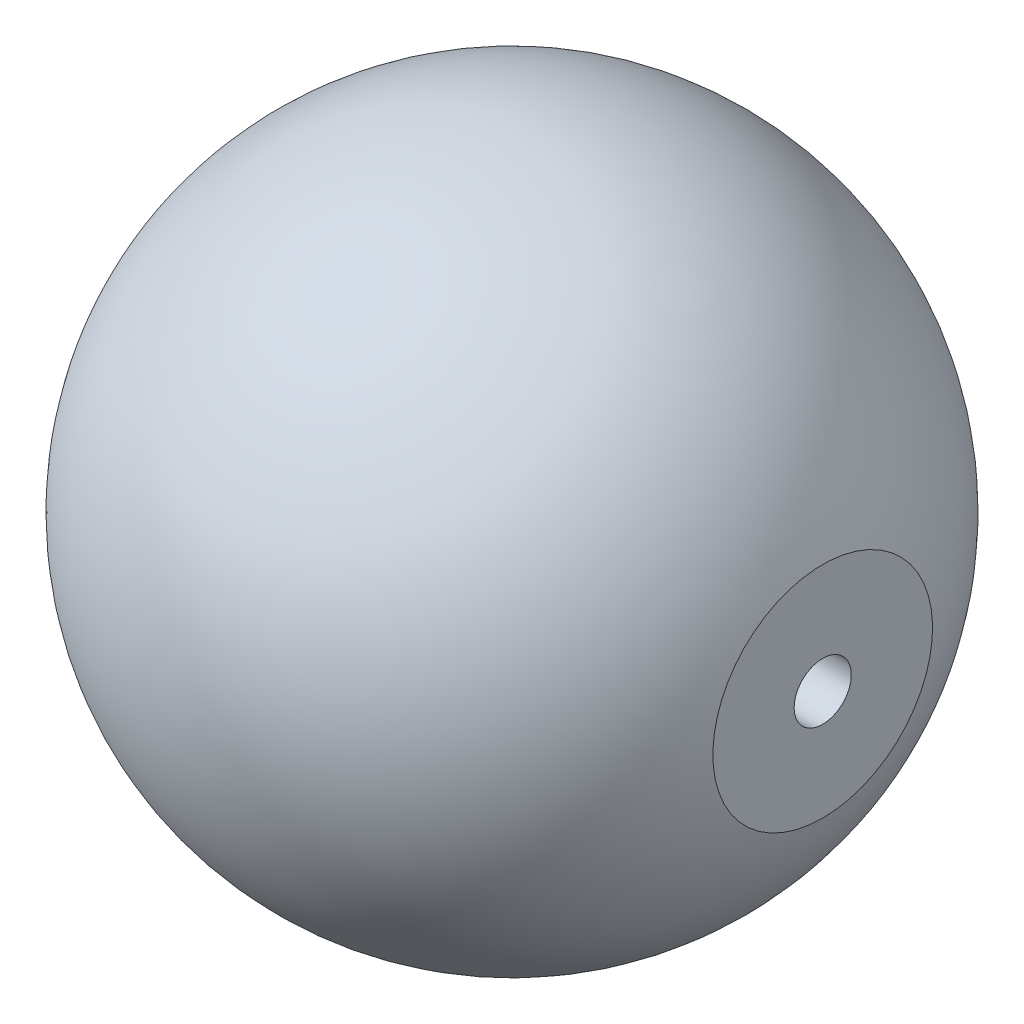
from build123d import *


with BuildPart() as part:
    # Knob Profile Sketch → Ball Knob Revolve (revolve)
    with BuildSketch(Plane.XY, mode=Mode.PRIVATE) as ball_knob_revolve_sk:
        with BuildLine():
            Line((-28.284271247, -2.6), (-28.284271247, -10))
            ThreePointArc((-28.284271247, -10), (0, -30), (28.284271247, -10))
            Line((28.284271247, -10), (28.284271247, -2.6))
            Line((28.284271247, -2.6), (-28.284271247, -2.6))
        make_face()
    revolve(ball_knob_revolve_sk.sketch.rotate(Axis((-30, 0, 0), (1, 0, 0)), 270), axis=Axis((-30, 0, 0), (1, 0, 0)))


solid = part.part
